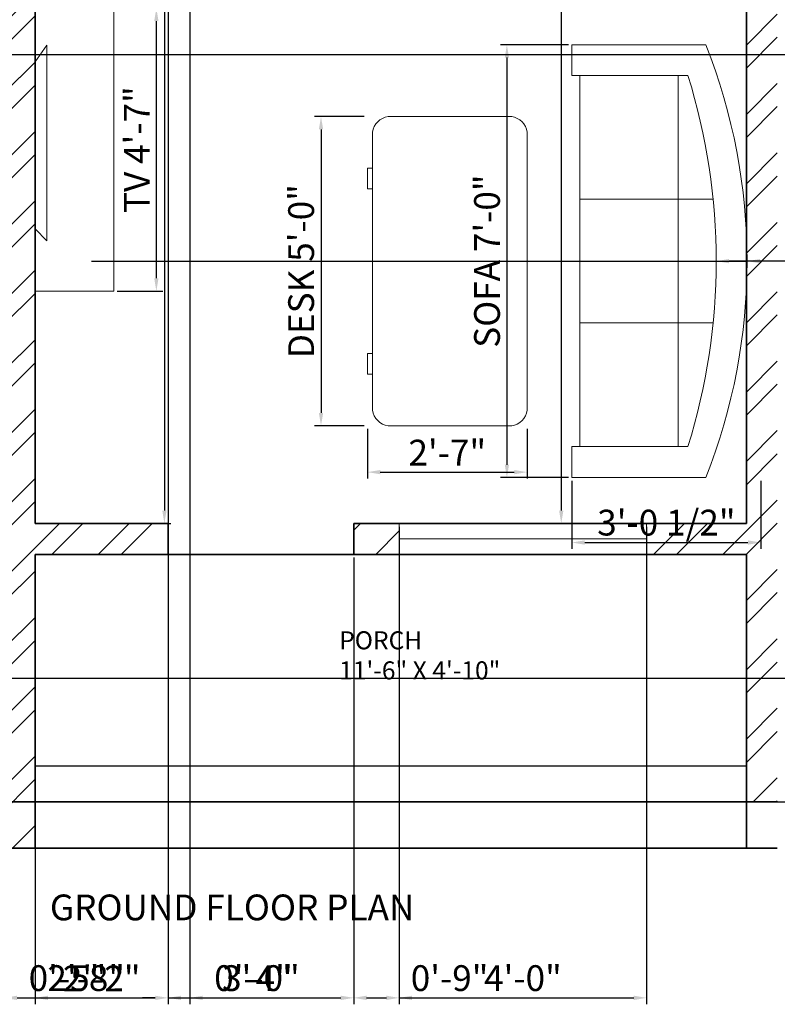
# Model space of a CAD drawing. Units: inches. Extents: x 28986 to 29505, y -162 to 451.
# Tile 2 of 6: x 29171 to 29318, y -159 to 32. Entities that reach past the tile are written whole.
import ezdxf

# ---------------------------------------------------------------- set-up
doc = ezdxf.new("R2010")
doc.units = ezdxf.units.IN
doc.layers.get('Defpoints').update_dxf_attribs({"color": 120})
doc.layers.add('A-ANNO-DIMS', color=9, linetype='Continuous', lineweight=18, true_color=0xafd9aa)
doc.layers.add('A-FLOR-STRS', color=32, linetype='Continuous', lineweight=25, true_color=0xcd6928)
for name, color, linetype, lineweight in [('A-ANNO-TITL', 3, 'Continuous', 25), ('A-AREA-IDEN', 6, 'Continuous', 18), ('A-EQPM', 8, 'Continuous', 18), ('A-GLAZ', 4, 'Continuous', 18), ('A-WALL', 7, 'Continuous', 35), ('A-WALL-PATT', 1, 'Continuous', 13), ('FURNITURE', 241, 'Continuous', 18)]:
    doc.layers.add(name, color=color, linetype=linetype, lineweight=lineweight)
doc.styles.get("Standard").update_dxf_attribs({"font": 'arial.ttf'})
doc.dimstyles.new('ISO-25', dxfattribs={"dimtxt": 5, "dimasz": 2.5, "dimexe": 1.25, "dimexo": 0.625, "dimtad": 1, "dimdec": 0, "dimlunit": 3, "dimtxsty": 'Standard', "dimcen": 2.5, "dimadec": 0, "dimazin": 0, "dimtfac": 1, "dimtdec": 0, "dimtmove": 0, "dimatfit": 3, "dimfxl": 1, "dimarcsym": 0})

# ---------------------------------------------------------------- blocks, each defined once
blk = doc.blocks.new('tv')
for p, q in [((18.34, 53.39), (15.62, 57.31)), ((15.62, 57.31), (15.62, 11.74)), ((15.62, 11.74), (18.34, 14.53))]:
    blk.add_line(p, q)
blk.add_lwpolyline([(18.34, 0), (0, 0), (0, 65.9), (18.34, 65.9)], close=True)
blk = doc.blocks.new('Desk - 30 x 60 in.')
for p, q in [((-26.999995, 0), (26.999995, 0)), ((-29.999995, -27), (-29.999995, -3)), ((29.999995, -3), (29.999995, -27)), ((26.999995, -30), (-26.999995, -30)), ((-20.000005, -30), (-20.000005, -31)), ((-16.000005, -31), (-16.000005, -30)), ((15.999995, -31), (15.999995, -30)), ((19.999995, -30), (19.999995, -31)), ((-20.000005, -31), (-16.000005, -31)), ((19.999995, -31), (15.999995, -31))]:
    blk.add_line(p, q)
for centre, start, end in [((-26.499995, -3.5), 98.1301, 171.8699), ((26.499995, -3.5), 8.130102, 81.8699), ((-26.499995, -26.5), 188.1301, 261.8699), ((26.499995, -26.5), 278.1301, 351.8699)]:
    blk.add_arc(centre, 3.535534, start, end)
blk = doc.blocks.new('Sofa - Roundback 7 ft.')
for p, q in [((-12.00002, -32.4421), (-12.00003, -6.5971)), ((11.99997, -32.4421), (11.99998, -6.5971)), ((-36.000027, -34), (-36.000027, -11.4696)), ((35.99998, -34), (35.99998, -11.4696)), ((-35.999844, -13.3819), (35.9998, -13.3819)), ((-36.000027, -32.4421), (35.99998, -32.4421))]:
    blk.add_line(p, q)
for points in [[(-36.000027, -34), (-42.000027, -34), (-42.000027, -8)], [(41.99998, -8), (41.99998, -34), (35.99998, -34)]]:
    blk.add_lwpolyline(points)
for centre, radius, start, end in [((0, -114.25), 114.25, 68.43141, 111.5686), ((-0.00001, -127.1968), 121.1968, 72.72033, 107.2797)]:
    blk.add_arc(centre, radius, start, end)
blk = doc.blocks.new('*D18')
at = {"layer": 'A-ANNO-DIMS', "color": 0, "lineweight": -2, "transparency": 16777216}
for p, q in [((29278.83, 326.7), (29274.99, 326.7)), ((29276.24, 324.2), (29276.24, -62.8)), ((29278.83, -65.3), (29274.99, -65.3))]:
    blk.add_line(p, q, dxfattribs=at)
at = {"layer": 'A-ANNO-DIMS', "color": 0, "transparency": 16777216}
for points in [[(29275.82, 324.2), (29276.65, 324.2), (29276.24, 326.7)], [(29275.82, -62.8), (29276.65, -62.8), (29276.24, -65.3)]]:
    blk.add_solid(points, dxfattribs=at)
at = {"layer": 'Defpoints', "color": 0, "transparency": 16777216}
for p in [(29279.46, 326.7), (29276.24, -65.3), (29279.46, -65.3)]:
    blk.add_point(p, dxfattribs=at)
at = {"layer": 'A-ANNO-DIMS', "color": 0, "transparency": 16777216, "insert": (29273.06, 130.7), "char_height": 5, "attachment_point": 5, "rotation": 90}
blk.add_mtext('32\'-8"', dxfattribs=at)
blk = doc.blocks.new('*D19')
at = {"layer": 'A-ANNO-DIMS', "color": 0, "lineweight": -2, "transparency": 16777216}
for p, q in [((29196.21, 162.7), (29200.48, 162.7)), ((29199.23, 160.2), (29199.23, -62.8)), ((29196.21, -65.3), (29200.48, -65.3))]:
    blk.add_line(p, q, dxfattribs=at)
at = {"layer": 'A-ANNO-DIMS', "color": 0, "transparency": 16777216}
for points in [[(29198.82, 160.2), (29199.65, 160.2), (29199.23, 162.7)], [(29198.82, -62.8), (29199.65, -62.8), (29199.23, -65.3)]]:
    blk.add_solid(points, dxfattribs=at)
at = {"layer": 'Defpoints', "color": 0, "transparency": 16777216}
for p in [(29195.59, 162.7), (29195.59, -65.3), (29199.23, -65.3)]:
    blk.add_point(p, dxfattribs=at)
at = {"layer": 'A-ANNO-DIMS', "color": 0, "transparency": 16777216, "insert": (29196.05, 48.7), "char_height": 5, "attachment_point": 5, "rotation": 90}
blk.add_mtext("19'", dxfattribs=at)
blk = doc.blocks.new('*D55')
at = {"layer": 'A-ANNO-DIMS', "color": 0, "lineweight": -2, "transparency": 16777216}
for p, q in [((29190.06, 34.7), (29198.93, 34.7)), ((29197.68, -17.72), (29197.68, 32.2)), ((29190.06, -20.22), (29198.93, -20.22))]:
    blk.add_line(p, q, dxfattribs=at)
at = {"layer": 'A-ANNO-DIMS', "color": 0, "transparency": 16777216}
for points in [[(29197.26, 32.2), (29198.09, 32.2), (29197.68, 34.7)], [(29197.26, -17.72), (29198.09, -17.72), (29197.68, -20.22)]]:
    blk.add_solid(points, dxfattribs=at)
at = {"layer": 'Defpoints', "color": 0, "transparency": 16777216}
for p in [(29189.44, 34.7), (29197.68, 34.7), (29189.44, -20.22)]:
    blk.add_point(p, dxfattribs=at)
at = {"layer": 'A-ANNO-DIMS', "color": 0, "transparency": 16777216, "insert": (29194.55, 7.24), "char_height": 5, "attachment_point": 5, "rotation": 90}
blk.add_mtext('TV 4\'-7"', dxfattribs=at)
blk = doc.blocks.new('*D57')
at = {"layer": 'A-ANNO-DIMS', "color": 0, "lineweight": -2, "transparency": 16777216}
for p, q in [((29277.67, 27.61), (29264.44, 27.61)), ((29265.69, 25.11), (29265.69, -53.89)), ((29277.67, -56.39), (29264.44, -56.39))]:
    blk.add_line(p, q, dxfattribs=at)
at = {"layer": 'A-ANNO-DIMS', "color": 0, "transparency": 16777216}
for points in [[(29265.28, 25.11), (29266.11, 25.11), (29265.69, 27.61)], [(29265.28, -53.89), (29266.11, -53.89), (29265.69, -56.39)]]:
    blk.add_solid(points, dxfattribs=at)
at = {"layer": 'Defpoints', "color": 0, "transparency": 16777216}
for p in [(29278.29, 27.61), (29265.69, -56.39), (29278.29, -56.39)]:
    blk.add_point(p, dxfattribs=at)
at = {"layer": 'A-ANNO-DIMS', "color": 0, "transparency": 16777216, "insert": (29262.48, -14.39), "char_height": 5, "attachment_point": 5, "rotation": 90}
blk.add_mtext('SOFA 7\'-0"', dxfattribs=at)
blk = doc.blocks.new('*D58')
at = {"layer": 'A-ANNO-DIMS', "color": 0, "lineweight": -2, "transparency": 16777216}
for p, q in [((29278.29, -57.02), (29278.29, -70.24)), ((29314.96, -57.02), (29314.96, -70.24)), ((29280.79, -68.99), (29312.46, -68.99))]:
    blk.add_line(p, q, dxfattribs=at)
at = {"layer": 'A-ANNO-DIMS', "color": 0, "transparency": 16777216}
for points in [[(29280.79, -68.58), (29280.79, -69.41), (29278.29, -68.99)], [(29312.46, -68.58), (29312.46, -69.41), (29314.96, -68.99)]]:
    blk.add_solid(points, dxfattribs=at)
at = {"layer": 'Defpoints', "color": 0, "transparency": 16777216}
for p in [(29278.29, -56.39), (29314.96, -56.39), (29314.96, -68.99)]:
    blk.add_point(p, dxfattribs=at)
at = {"layer": 'A-ANNO-DIMS', "color": 0, "transparency": 16777216, "insert": (29296.63, -65.78), "char_height": 5, "attachment_point": 5}
blk.add_mtext('3\'-0 1/2"', dxfattribs=at)
blk = doc.blocks.new('*D59')
at = {"layer": 'A-ANNO-DIMS', "color": 0, "lineweight": -2, "transparency": 16777216}
for p, q in [((29238, 13.66), (29228.37, 13.66)), ((29229.62, 11.16), (29229.62, -43.84)), ((29238, -46.34), (29228.37, -46.34))]:
    blk.add_line(p, q, dxfattribs=at)
at = {"layer": 'A-ANNO-DIMS', "color": 0, "transparency": 16777216}
for points in [[(29229.21, 11.16), (29230.04, 11.16), (29229.62, 13.66)], [(29229.21, -43.84), (29230.04, -43.84), (29229.62, -46.34)]]:
    blk.add_solid(points, dxfattribs=at)
at = {"layer": 'Defpoints', "color": 0, "transparency": 16777216}
for p in [(29238.62, 13.66), (29229.62, -46.34), (29238.62, -46.34)]:
    blk.add_point(p, dxfattribs=at)
at = {"layer": 'A-ANNO-DIMS', "color": 0, "transparency": 16777216, "insert": (29226.41, -16.34), "char_height": 5, "attachment_point": 5, "rotation": 90}
blk.add_mtext('DESK 5\'-0"', dxfattribs=at)
blk = doc.blocks.new('*D60')
at = {"layer": 'A-ANNO-DIMS', "color": 0, "lineweight": -2, "transparency": 16777216}
for p, q in [((29238.62, -46.96), (29238.62, -56.59)), ((29269.62, -46.96), (29269.62, -56.59)), ((29241.12, -55.34), (29267.12, -55.34))]:
    blk.add_line(p, q, dxfattribs=at)
at = {"layer": 'A-ANNO-DIMS', "color": 0, "transparency": 16777216}
for points in [[(29241.12, -54.92), (29241.12, -55.75), (29238.62, -55.34)], [(29267.12, -54.92), (29267.12, -55.75), (29269.62, -55.34)]]:
    blk.add_solid(points, dxfattribs=at)
at = {"layer": 'Defpoints', "color": 0, "transparency": 16777216}
for p in [(29238.62, -46.34), (29269.62, -46.34), (29269.62, -55.34)]:
    blk.add_point(p, dxfattribs=at)
at = {"layer": 'A-ANNO-DIMS', "color": 0, "transparency": 16777216, "insert": (29254.12, -52.2), "char_height": 5, "attachment_point": 5}
blk.add_mtext('2\'-7"', dxfattribs=at)
blk = doc.blocks.new('*D65')
at = {"layer": 'A-ANNO-DIMS', "color": 0, "lineweight": -2, "transparency": 16777216}
for p, q in [((29168.78, 25.7), (29501.46, 25.7)), ((29500.21, -116.8), (29500.21, 23.2)), ((29168.78, -119.3), (29501.46, -119.3))]:
    blk.add_line(p, q, dxfattribs=at)
at = {"layer": 'A-ANNO-DIMS', "color": 0, "transparency": 16777216}
for points in [[(29499.79, 23.2), (29500.62, 23.2), (29500.21, 25.7)], [(29499.79, -116.8), (29500.62, -116.8), (29500.21, -119.3)]]:
    blk.add_solid(points, dxfattribs=at)
at = {"layer": 'Defpoints', "color": 0, "transparency": 16777216}
for p in [(29168.16, 25.7), (29500.21, 25.7), (29168.16, -119.3)]:
    blk.add_point(p, dxfattribs=at)
at = {"layer": 'A-ANNO-DIMS', "color": 0, "transparency": 16777216, "insert": (29497.07, -46.8), "char_height": 5, "attachment_point": 5, "rotation": 90}
blk.add_mtext('12\'-1"', dxfattribs=at)
blk = doc.blocks.new('*D74')
at = {"layer": 'A-ANNO-DIMS', "color": 0, "lineweight": -2, "transparency": 16777216}
for p, q in [((29199.96, -71.93), (29199.96, -158.6)), ((29235.96, -71.93), (29235.96, -158.6)), ((29202.46, -157.35), (29233.46, -157.35))]:
    blk.add_line(p, q, dxfattribs=at)
at = {"layer": 'A-ANNO-DIMS', "color": 0, "transparency": 16777216}
for points in [[(29202.46, -156.93), (29202.46, -157.77), (29199.96, -157.35)], [(29233.46, -156.93), (29233.46, -157.77), (29235.96, -157.35)]]:
    blk.add_solid(points, dxfattribs=at)
at = {"layer": 'Defpoints', "color": 0, "transparency": 16777216}
for p in [(29199.96, -71.3), (29235.96, -71.3), (29235.96, -157.35)]:
    blk.add_point(p, dxfattribs=at)
at = {"layer": 'A-ANNO-DIMS', "color": 0, "transparency": 16777216, "insert": (29217.96, -154.17), "char_height": 5, "attachment_point": 5}
blk.add_mtext('3\'-0"', dxfattribs=at)
blk = doc.blocks.new('*D75')
at = {"layer": 'A-ANNO-DIMS', "color": 0, "lineweight": -2, "transparency": 16777216}
for p, q in [((29174.16, -71.93), (29174.16, -158.6)), ((29199.96, -71.93), (29199.96, -158.6)), ((29176.66, -157.35), (29197.46, -157.35))]:
    blk.add_line(p, q, dxfattribs=at)
at = {"layer": 'A-ANNO-DIMS', "color": 0, "transparency": 16777216}
for points in [[(29176.66, -156.93), (29176.66, -157.77), (29174.16, -157.35)], [(29197.46, -156.93), (29197.46, -157.77), (29199.96, -157.35)]]:
    blk.add_solid(points, dxfattribs=at)
at = {"layer": 'Defpoints', "color": 0, "transparency": 16777216}
for p in [(29174.16, -71.3), (29199.96, -71.3), (29199.96, -157.35)]:
    blk.add_point(p, dxfattribs=at)
at = {"layer": 'A-ANNO-DIMS', "color": 0, "transparency": 16777216, "insert": (29187.06, -154.22), "char_height": 5, "attachment_point": 5}
blk.add_mtext('2\'-2"', dxfattribs=at)
blk = doc.blocks.new('*D76')
at = {"layer": 'A-ANNO-DIMS', "color": 0, "lineweight": -2, "transparency": 16777216}
for p, q in [((29244.8, -65.93), (29244.8, -158.6)), ((29235.96, -71.93), (29235.96, -158.6)), ((29238.46, -157.35), (29242.3, -157.35)), ((29244.8, -157.35), (29261.84, -157.35))]:
    blk.add_line(p, q, dxfattribs=at)
at = {"layer": 'A-ANNO-DIMS', "color": 0, "transparency": 16777216}
for points in [[(29238.46, -156.93), (29238.46, -157.77), (29235.96, -157.35)], [(29242.3, -156.93), (29242.3, -157.77), (29244.8, -157.35)]]:
    blk.add_solid(points, dxfattribs=at)
at = {"layer": 'Defpoints', "color": 0, "transparency": 16777216}
for p in [(29244.8, -65.3), (29235.96, -71.3), (29244.8, -157.35)]:
    blk.add_point(p, dxfattribs=at)
at = {"layer": 'A-ANNO-DIMS', "color": 0, "transparency": 16777216, "insert": (29254.57, -154.17), "char_height": 5, "attachment_point": 5}
blk.add_mtext('0\'-9"', dxfattribs=at)
blk = doc.blocks.new('*D77')
at = {"layer": 'A-ANNO-DIMS', "color": 0, "lineweight": -2, "transparency": 16777216}
for p, q in [((29244.8, -65.93), (29244.8, -158.6)), ((29292.8, -65.93), (29292.8, -158.6)), ((29247.3, -157.35), (29290.3, -157.35))]:
    blk.add_line(p, q, dxfattribs=at)
at = {"layer": 'A-ANNO-DIMS', "color": 0, "transparency": 16777216}
for points in [[(29247.3, -156.93), (29247.3, -157.77), (29244.8, -157.35)], [(29290.3, -156.93), (29290.3, -157.77), (29292.8, -157.35)]]:
    blk.add_solid(points, dxfattribs=at)
at = {"layer": 'Defpoints', "color": 0, "transparency": 16777216}
for p in [(29244.8, -65.3), (29292.8, -65.3), (29292.8, -157.35)]:
    blk.add_point(p, dxfattribs=at)
at = {"layer": 'A-ANNO-DIMS', "color": 0, "transparency": 16777216, "insert": (29268.8, -154.17), "char_height": 5, "attachment_point": 5}
blk.add_mtext('4\'-0"', dxfattribs=at)
blk = doc.blocks.new('*D83')
at = {"layer": 'A-ANNO-DIMS', "color": 0, "lineweight": -2, "transparency": 16777216}
for p, q in [((29163.04, 25.07), (29163.04, -158.6)), ((29168.16, 25.07), (29168.16, -158.6)), ((29160.54, -157.35), (29158.04, -157.35)), ((29163.04, -157.35), (29168.16, -157.35)), ((29170.66, -157.35), (29187.7, -157.35))]:
    blk.add_line(p, q, dxfattribs=at)
at = {"layer": 'A-ANNO-DIMS', "color": 0, "transparency": 16777216}
for points in [[(29160.54, -156.93), (29160.54, -157.77), (29163.04, -157.35)], [(29170.66, -156.93), (29170.66, -157.77), (29168.16, -157.35)]]:
    blk.add_solid(points, dxfattribs=at)
at = {"layer": 'Defpoints', "color": 0, "transparency": 16777216}
for p in [(29163.04, 25.7), (29168.16, 25.7), (29168.16, -157.35)]:
    blk.add_point(p, dxfattribs=at)
at = {"layer": 'A-ANNO-DIMS', "color": 0, "transparency": 16777216, "insert": (29180.43, -154.17), "char_height": 5, "attachment_point": 5}
blk.add_mtext('0\'-5"', dxfattribs=at)
blk = doc.blocks.new('*D84')
at = {"layer": 'A-ANNO-DIMS', "color": 0, "lineweight": -2, "transparency": 16777216}
for p, q in [((29168.16, 162.07), (29168.16, -158.6)), ((29199.96, 162.07), (29199.96, -158.6)), ((29170.66, -157.35), (29197.46, -157.35))]:
    blk.add_line(p, q, dxfattribs=at)
at = {"layer": 'A-ANNO-DIMS', "color": 0, "transparency": 16777216}
for points in [[(29170.66, -156.93), (29170.66, -157.77), (29168.16, -157.35)], [(29197.46, -156.93), (29197.46, -157.77), (29199.96, -157.35)]]:
    blk.add_solid(points, dxfattribs=at)
at = {"layer": 'Defpoints', "color": 0, "transparency": 16777216}
for p in [(29168.16, 162.7), (29199.96, 162.7), (29199.96, -157.35)]:
    blk.add_point(p, dxfattribs=at)
at = {"layer": 'A-ANNO-DIMS', "color": 0, "transparency": 16777216, "insert": (29184.06, -154.17), "char_height": 5, "attachment_point": 5}
blk.add_mtext('2\'-8"', dxfattribs=at)
blk = doc.blocks.new('*D89')
at = {"layer": 'A-ANNO-DIMS', "color": 0, "lineweight": -2, "transparency": 16777216}
for p, q in [((29084.78, -95.3), (29501.46, -95.3)), ((29500.21, -97.8), (29500.21, -116.8)), ((29084.78, -119.3), (29501.46, -119.3))]:
    blk.add_line(p, q, dxfattribs=at)
at = {"layer": 'A-ANNO-DIMS', "color": 0, "transparency": 16777216}
for points in [[(29499.79, -97.8), (29500.62, -97.8), (29500.21, -95.3)], [(29499.79, -116.8), (29500.62, -116.8), (29500.21, -119.3)]]:
    blk.add_solid(points, dxfattribs=at)
at = {"layer": 'Defpoints', "color": 0, "transparency": 16777216}
for p in [(29084.16, -95.3), (29084.16, -119.3), (29500.21, -119.3)]:
    blk.add_point(p, dxfattribs=at)
at = {"layer": 'A-ANNO-DIMS', "color": 0, "transparency": 16777216, "insert": (29497.03, -107.3), "char_height": 5, "attachment_point": 5, "rotation": 90}
blk.add_mtext('2\'-0"', dxfattribs=at)
blk = doc.blocks.new('*D98')
at = {"layer": 'A-ANNO-DIMS', "color": 0, "lineweight": -2, "transparency": 16777216}
for p, q in [((29204.16, 168.07), (29204.16, -158.6)), ((29199.96, 162.07), (29199.96, -158.6)), ((29197.46, -157.35), (29194.96, -157.35)), ((29199.96, -157.35), (29204.16, -157.35)), ((29206.66, -157.35), (29223.7, -157.35))]:
    blk.add_line(p, q, dxfattribs=at)
at = {"layer": 'A-ANNO-DIMS', "color": 0, "transparency": 16777216}
for points in [[(29197.46, -156.93), (29197.46, -157.77), (29199.96, -157.35)], [(29206.66, -156.93), (29206.66, -157.77), (29204.16, -157.35)]]:
    blk.add_solid(points, dxfattribs=at)
at = {"layer": 'Defpoints', "color": 0, "transparency": 16777216}
for p in [(29204.16, 168.7), (29199.96, 162.7), (29204.16, -157.35)]:
    blk.add_point(p, dxfattribs=at)
at = {"layer": 'A-ANNO-DIMS', "color": 0, "transparency": 16777216, "insert": (29216.43, -154.17), "char_height": 5, "attachment_point": 5}
blk.add_mtext('0\'-4"', dxfattribs=at)
blk = doc.blocks.new('*D99')
at = {"layer": 'A-ANNO-DIMS', "color": 0, "lineweight": -2, "transparency": 16777216}
for p, q in [((29185.1, -14.39), (29306.29, -14.39)), ((29390.62, -14.39), (29308.79, -14.39))]:
    blk.add_line(p, q, dxfattribs=at)
at = {"layer": 'A-ANNO-DIMS', "color": 0, "transparency": 16777216}
blk.add_solid([(29308.79, -13.98), (29308.79, -14.81), (29306.29, -14.39)], dxfattribs=at)
at = {"layer": 'Defpoints', "color": 0, "transparency": 16777216}
for p in [(29185.1, -14.39), (29306.29, -14.39)]:
    blk.add_point(p, dxfattribs=at)
at = {"layer": 'A-ANNO-DIMS', "color": 0, "transparency": 16777216, "insert": (29379.01, -11.22), "char_height": 5, "attachment_point": 5, "rotation": 0}
blk.add_mtext('R10\'-1"', dxfattribs=at)
blk = doc.blocks.new('*D100')
at = {"layer": 'A-ANNO-DIMS', "color": 0, "lineweight": -2, "transparency": 16777216}
for p, q in [((29198.04, -14.39), (29312.29, -14.39)), ((29396.33, -14.39), (29314.79, -14.39))]:
    blk.add_line(p, q, dxfattribs=at)
at = {"layer": 'A-ANNO-DIMS', "color": 0, "transparency": 16777216}
blk.add_solid([(29314.79, -13.98), (29314.79, -14.81), (29312.29, -14.39)], dxfattribs=at)
at = {"layer": 'Defpoints', "color": 0, "transparency": 16777216}
for p in [(29198.04, -14.39), (29312.29, -14.39)]:
    blk.add_point(p, dxfattribs=at)
at = {"layer": 'A-ANNO-DIMS', "color": 0, "transparency": 16777216, "insert": (29380.84, -11.18), "char_height": 5, "attachment_point": 5, "rotation": 0}
blk.add_mtext('R9\'-6 1/2"', dxfattribs=at)

msp = doc.modelspace()

# ---------------------------------------------------------------- hatches: boundary and pattern name
at = {"layer": 'A-WALL-PATT'}
h = msp.add_hatch(dxfattribs=at)
h.set_pattern_fill('ANSI32', color=256)
h.paths.add_polyline_path([(29174.16, 34.7), (29163.04, 34.7), (29163.04, 29.3), (29163.04, 25.7), (29168.16, 25.7), (29168.16, -119.3), (29174.16, -119.3), (29174.16, -71.3), (29199.96, -71.3), (29199.96, -65.3), (29174.16, -65.3)])
h.paths.add_polyline_path([(29244.8, -65.3), (29235.96, -65.3), (29235.96, -71.3), (29244.8, -71.3)])
h.paths.add_polyline_path([(29318.16, 39.7), (29462.16, 39.7), (29462.16, 44.7), (29318.16, 44.7), (29318.16, 131.49), (29312.16, 131.49), (29312.16, -65.3), (29292.8, -65.3), (29292.8, -71.3), (29312.16, -71.3), (29312.16, -119.3), (29318.16, -119.3)])
h.paths.add_polyline_path([(29219.6, 411.7), (29051.16, 411.7), (29051.16, 368.84), (29060.16, 368.84), (29060.16, 402.7), (29204.16, 402.7), (29219.6, 402.7)])
h.paths.add_polyline_path([(29060.16, 320.84), (29051.16, 320.84), (29051.16, 231.24), (29060.16, 231.24), (29060.16, 252.7)])
h.paths.add_polyline_path([(29210.16, 265.69), (29204.76, 265.69), (29204.16, 265.69), (29204.16, 258.7), (29060.16, 258.7), (29060.16, 252.7), (29204.16, 252.7), (29204.16, 228.7), (29204.16, 168.7), (29199.96, 168.7), (29199.96, 167.47), (29199.96, 162.7), (29210.16, 162.7)])
h.paths.add_polyline_path([(29060.16, 183.24), (29051.16, 183.24), (29051.16, 162.7), (29060.16, 162.7), (29168.16, 162.7), (29168.16, 167.47), (29168.16, 168.7), (29060.16, 168.7)])
h.paths.add_polyline_path([(29060.16, 126.7), (29051.16, 126.7), (29051.16, 70.7), (29060.16, 70.7)])
h.paths.add_polyline_path([(29060.16, 25.7), (29127.04, 25.7), (29127.04, 34.7), (29060.16, 34.7), (29051.16, 34.7), (29051.16, -22.45), (29060.16, -22.45)])
h.paths.add_polyline_path([(29060.16, -70.45), (29051.16, -70.45), (29051.16, -128.3), (29084.16, -128.3), (29084.16, -119.3), (29060.16, -119.3)])
h.paths.add_polyline_path([(29174.16, -119.3), (29168.16, -119.3), (29132.16, -119.3), (29132.16, -128.3), (29174.16, -128.3)])
h.paths.add_polyline_path([(29471.16, 79.78), (29462.16, 79.78), (29462.16, -119.3), (29462.16, -128.3), (29471.16, -128.3)])
h.paths.add_polyline_path([(29462.16, 182.7), (29318.16, 182.7), (29318.16, 191.79), (29317.56, 191.79), (29312.16, 191.79), (29312.16, 167.49), (29317.56, 167.49), (29318.16, 167.49), (29318.16, 176.7), (29462.16, 176.7)])
h.paths.add_polyline_path([(29471.16, 221.37), (29462.16, 221.37), (29462.16, 135.64), (29471.16, 135.64)])
h.paths.add_polyline_path([(29471.16, 360.33), (29462.16, 360.33), (29462.16, 277.22), (29471.16, 277.22)])
h.paths.add_polyline_path([(29471.16, 411.7), (29243.6, 411.7), (29243.6, 402.7), (29462.16, 402.7), (29462.16, 384.33), (29471.16, 384.33)])
h.paths.add_polyline_path([(29348.16, 402.7), (29342.16, 402.7), (29342.16, 332.7), (29308.66, 332.7), (29308.66, 326.7), (29312.16, 326.7), (29312.16, 227.79), (29318.16, 227.79), (29318.16, 326.7), (29355.99, 326.7), (29355.99, 332.7), (29348.16, 332.7)])
h.paths.add_polyline_path([(29210.16, 326.7), (29272.66, 326.7), (29272.66, 332.1), (29272.66, 332.7), (29210.16, 332.7), (29210.16, 402.7), (29204.16, 402.7), (29204.16, 316.6), (29204.16, 301.69), (29210.16, 301.69)])

# ---------------------------------------------------------------- linework, layer by layer
at = {"layer": 'A-FLOR-STRS'}
msp.add_line((29174.16, -112.3), (29312.16, -112.3), dxfattribs=at)
msp.add_lwpolyline([(29174.16, -119.3), (29312.16, -119.3)], dxfattribs=at)
at = {"layer": 'A-GLAZ'}
for p, q in [((29244.8, -65.3), (29244.8, -71.3)), ((29292.8, -65.3), (29292.8, -71.3)), ((29244.8, -68.3), (29292.8, -68.3))]:
    msp.add_line(p, q, dxfattribs=at)
at = {"layer": 'A-WALL'}
for p, q in [((29312.16, 326.7), (29312.16, -65.3)), ((29199.96, -65.3), (29174.16, -65.3)), ((29199.96, -65.3), (29199.96, -71.3)), ((29312.16, -65.3), (29235.96, -65.3)), ((29235.96, -65.3), (29235.96, -71.3)), ((29312.16, -71.3), (29174.16, -71.3)), ((29312.16, -71.3), (29312.16, -128.3)), ((29312.16, -71.3), (29312.16, -112.3)), ((29060.16, -119.3), (29318.16, -119.3)), ((29051.16, -128.3), (29318.16, -128.3))]:
    msp.add_line(p, q, dxfattribs=at)
for points in [[(29174.16, 34.7), (29174.16, -65.3)], [(29174.16, -71.3), (29174.16, -128.3)], [(29174.16, -71.3), (29174.16, -112.3)]]:
    msp.add_lwpolyline(points, dxfattribs=at)

# ---------------------------------------------------------------- block references
at = {"layer": 'A-EQPM', "xscale": -0.8333519629623783, "yscale": 0.8333519629623783, "zscale": 0.8333519629623783}
msp.add_blockref('tv', (29189.44, -20.22), dxfattribs=at)
at = {"layer": 'FURNITURE', "rotation": 270}
for name, p in [('Sofa - Roundback 7 ft.', (29312.29, -14.39)), ('Desk - 30 x 60 in.', (29269.62, -16.34))]:
    msp.add_blockref(name, p, dxfattribs=at)

# ---------------------------------------------------------------- texts
at = {"layer": 'A-ANNO-TITL', "insert": (29177.02, -137.3), "char_height": 5, "attachment_point": 1}
msp.add_mtext_dynamic_manual_height_columns('GROUND FLOOR PLAN', width=146.5558, gutter_width=12.5, heights=[0], dxfattribs=at)
at = {"layer": 'A-AREA-IDEN', "insert": (29233.14, -86.22), "char_height": 3.5, "attachment_point": 1}
msp.add_mtext_dynamic_manual_height_columns('PORCH\\P11\'-6" X 4\'-10"', width=65.867, gutter_width=12.5, heights=[0], dxfattribs=at)

# ---------------------------------------------------------------- dimensions: what is measured, and where the dimension line sits
at = {"layer": 'A-ANNO-DIMS'}
for base, p1, p2, override, picture, middle in [((29276.24, -65.3), (29279.46, 326.7), (29279.46, -65.3), {"dimclrd": 0, "dimclre": 0, "dimclrt": 0}, '*D18', (29273.06, 130.7)), ((29199.23, -65.3), (29195.59, 162.7), (29195.59, -65.3), {"dimclrd": 0, "dimclre": 0, "dimclrt": 0}, '*D19', (29196.05, 48.7)), ((29500.21, 25.7), (29168.16, -119.3), (29168.16, 25.7), {"dimdec": 1, "dimlfac": 1, "dimrnd": 0, "dimzin": 1, "dimdsep": 46, "dimlunit": 4, "dimfrac": 2}, '*D65', (29497.07, -46.8)), ((29500.21, -119.3), (29084.16, -95.3), (29084.16, -119.3), {"dimdec": 1, "dimlfac": 1, "dimrnd": 0, "dimzin": 1, "dimdsep": 46, "dimlunit": 4, "dimfrac": 2}, '*D89', (29497.03, -107.3))]:
    dim = msp.add_linear_dim(base=base, p1=p1, p2=p2, angle=90, dimstyle='ISO-25', override=override, dxfattribs=at)
    dim.commit()
    dim.dimension.update_dxf_attribs({"geometry": picture, "text_midpoint": middle})
for base, p1, p2, picture, middle in [((29204.16, -157.35), (29199.96, 162.7), (29204.16, 168.7), '*D98', (29216.43, -154.17)), ((29199.96, -157.35), (29168.16, 162.7), (29199.96, 162.7), '*D84', (29184.06, -154.17)), ((29168.16, -157.35), (29163.04, 25.7), (29168.16, 25.7), '*D83', (29180.43, -154.17)), ((29269.62, -55.34), (29238.62, -46.34), (29269.62, -46.34), '*D60', (29254.12, -52.2)), ((29314.96, -68.99), (29278.29, -56.39), (29314.96, -56.39), '*D58', (29296.63, -65.78)), ((29244.8, -157.35), (29235.96, -71.3), (29244.8, -65.3), '*D76', (29254.57, -154.17)), ((29292.8, -157.35), (29244.8, -65.3), (29292.8, -65.3), '*D77', (29268.8, -154.17)), ((29199.96, -157.35), (29174.16, -71.3), (29199.96, -71.3), '*D75', (29187.06, -154.22)), ((29235.96, -157.35), (29199.96, -71.3), (29235.96, -71.3), '*D74', (29217.96, -154.17))]:
    dim = msp.add_linear_dim(base=base, p1=p1, p2=p2, dimstyle='ISO-25', override={"dimdec": 1, "dimlfac": 1, "dimrnd": 0, "dimzin": 1, "dimdsep": 46, "dimlunit": 4, "dimfrac": 2}, dxfattribs=at)
    dim.commit()
    dim.dimension.update_dxf_attribs({"geometry": picture, "text_midpoint": middle})
for base, p1, p2, angle, text, picture, middle in [((29197.68, 34.7), (29189.44, -20.22), (29189.44, 34.7), 90, 'TV <>', '*D55', (29194.55, 7.24)), ((29265.69, -56.39), (29278.29, 27.61), (29278.29, -56.39), 270, 'SOFA <>', '*D57', (29262.48, -14.39)), ((29229.62, -46.34), (29238.62, 13.66), (29238.62, -46.34), 270, 'DESK <>', '*D59', (29226.41, -16.34))]:
    dim = msp.add_linear_dim(base=base, p1=p1, p2=p2, angle=angle, text=text, dimstyle='ISO-25', override={"dimdec": 1, "dimlfac": 1, "dimrnd": 0, "dimzin": 1, "dimdsep": 46, "dimlunit": 4, "dimfrac": 2}, dxfattribs=at)
    dim.commit()
    dim.dimension.update_dxf_attribs({"geometry": picture, "text_midpoint": middle})
for center, mpoint, picture, middle in [((29198.044791, -14.394047), (29312.294791, -14.394), '*D100', (29380.844791, -14.3939718)), ((29185.1, -14.39), (29306.29, -14.39), '*D99', (29379.01, -14.39))]:
    dim = msp.add_radius_dim(center=center, mpoint=mpoint, dimstyle='ISO-25', override={"dimdec": 1, "dimlfac": 1, "dimrnd": 0, "dimzin": 1, "dimdsep": 46, "dimlunit": 4, "dimfrac": 2}, dxfattribs=at)
    dim.commit()
    dim.dimension.update_dxf_attribs({"geometry": picture, "text_midpoint": middle, "dimtype": 164})

doc.saveas('drawing.dxf')
